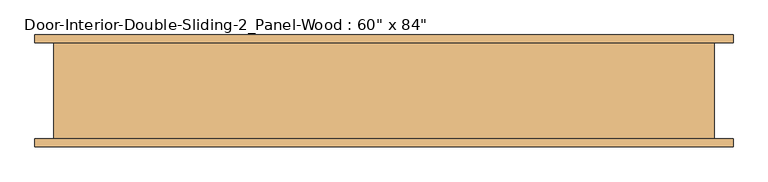
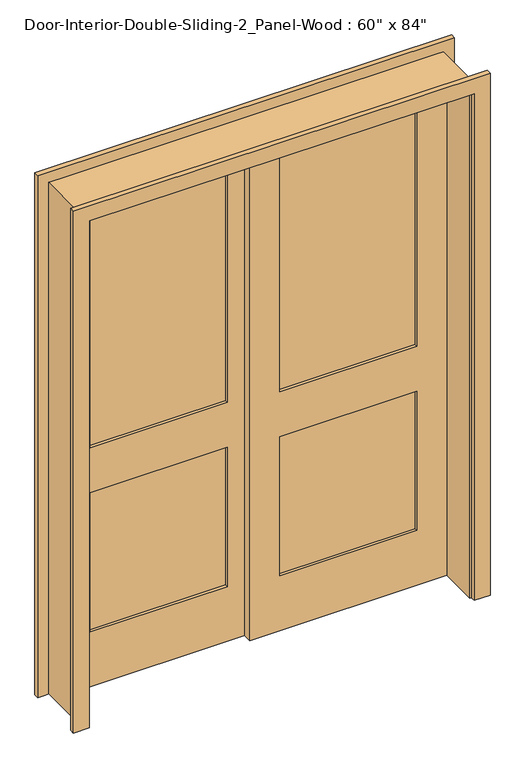
"""IFC4 building model written with IfcOpenShell, lengths in millimetres: door geometry."""

from ifc_helpers import new_model, si_unit, frame, origin, place, context, project, spatial, polyline, outline, extrude, source, transform, mapped, element, save


def door_2b3f2951(model_context):
    return source(origin(), model_context, "Body", "SweptSolid", [
        extrude(outline(polyline([(0.0, 762.0), (0.0, 787.4), (2159.0, 787.4), (2159.0, -787.4), (0.0, -787.4), (0.0, -762.0), (2133.6, -762.0), (2133.6, 762.0), (0.0, 762.0)])), frame((0.0, -117.475, 0.0), z_axis=(0.0, 1.0, 0.0), x_axis=(0.0, 0.0, 1.0)), (0.0, 0.0, 1.0), 228.6),
        extrude(outline(polyline([(2133.6, -762.0), (0.0, -762.0), (0.0, 25.4), (2133.6, 25.4), (2133.6, -762.0)]), holes=[polyline([(2014.5375, -641.35), (2014.5375, -95.25), (1009.65, -95.25), (1009.65, -641.35), (2014.5375, -641.35)]), polyline([(819.15, -641.35), (819.15, -95.25), (231.775, -95.25), (231.775, -641.35), (819.15, -641.35)])]), frame((0.0, 76.2, 0.0), z_axis=(0.0, 1.0, 0.0), x_axis=(0.0, 0.0, 1.0)), (0.0, 0.0, 1.0), 34.925),
        extrude(outline(polyline([(-95.25, 87.8416667), (-641.35, 87.8416667), (-641.35, 99.4833333), (-95.25, 99.4833333), (-95.25, 87.8416667)])), frame((0.0, 0.0, 1009.65), z_axis=(0.0, 0.0, 1.0), x_axis=(1.0, 0.0, 0.0)), (0.0, 0.0, 1.0), 1004.8875),
        extrude(outline(polyline([(-95.25, 87.8416667), (-641.35, 87.8416667), (-641.35, 99.4833333), (-95.25, 99.4833333), (-95.25, 87.8416667)])), frame((0.0, 0.0, 231.775), z_axis=(0.0, 0.0, 1.0), x_axis=(1.0, 0.0, 0.0)), (0.0, 0.0, 1.0), 587.375),
        extrude(outline(polyline([(2133.6, -25.4), (0.0, -25.4), (0.0, 762.0), (2133.6, 762.0), (2133.6, -25.4)]), holes=[polyline([(2014.5375, 95.25), (2014.5375, 641.35), (1009.65, 641.35), (1009.65, 95.25), (2014.5375, 95.25)]), polyline([(819.15, 95.25), (819.15, 641.35), (231.775, 641.35), (231.775, 95.25), (819.15, 95.25)])]), frame((0.0, 41.275, 0.0), z_axis=(0.0, 1.0, 0.0), x_axis=(0.0, 0.0, 1.0)), (0.0, 0.0, 1.0), 34.925),
        extrude(outline(polyline([(641.35, 52.9166667), (95.25, 52.9166667), (95.25, 64.5583333), (641.35, 64.5583333), (641.35, 52.9166667)])), frame((0.0, 0.0, 1009.65), z_axis=(0.0, 0.0, 1.0), x_axis=(1.0, 0.0, 0.0)), (0.0, 0.0, 1.0), 1004.8875),
        extrude(outline(polyline([(641.35, 52.9166667), (95.25, 52.9166667), (95.25, 64.5583333), (641.35, 64.5583333), (641.35, 52.9166667)])), frame((0.0, 0.0, 231.775), z_axis=(0.0, 0.0, 1.0), x_axis=(1.0, 0.0, 0.0)), (0.0, 0.0, 1.0), 587.375),
        extrude(outline(polyline([(0.0, 768.35), (0.0, 831.85), (2203.45, 831.85), (2203.45, -831.85), (0.0, -831.85), (0.0, -768.35), (2139.95, -768.35), (2139.95, 768.35), (0.0, 768.35)])), frame((0.0, 111.125, 0.0), z_axis=(0.0, 1.0, 0.0), x_axis=(0.0, 0.0, 1.0)), (0.0, 0.0, 1.0), 19.05),
        extrude(outline(polyline([(0.0, 768.35), (0.0, 831.85), (2203.45, 831.85), (2203.45, -831.85), (0.0, -831.85), (0.0, -768.35), (2139.95, -768.35), (2139.95, 768.35), (0.0, 768.35)])), frame((0.0, -136.525, 0.0), z_axis=(0.0, 1.0, 0.0), x_axis=(0.0, 0.0, 1.0)), (0.0, 0.0, 1.0), 19.05),
    ])


if __name__ == "__main__":
    model = new_model("IFC4")
    model_context = context("Model", 3, world=origin())
    ifc_project = project(units=[si_unit("LENGTHUNIT", "METRE", prefix="MILLI")], contexts=[model_context])
    site = spatial("IfcSite", under=ifc_project)
    building = spatial("IfcBuilding", under=site)
    placement = place(None, origin())
    door_shape = door_2b3f2951(model_context)
    element("IfcDoor", 1, ObjectType="Door-Interior-Double-Sliding-2_Panel-Wood : 60\" x 84\"", at=placement, inside=building, context=model_context, shape_type="MappedRepresentation", body=[
        mapped(door_shape, transform((0.0, 0.0, 0.0), x_axis=(1.0, 0.0, 0.0), y_axis=(0.0, 1.0, 0.0), z_axis=(0.0, 0.0, 1.0))),
    ])
    save(model, "model.ifc")

# Revit data of these elements
# Type "Door-Interior-Double-Sliding-2_Panel-Wood : 60\" x 84\""
#   Type Mark = "10"
#   Assembly Code = "C1020300"
#   Analytic Construction = "Wooden"
#   Top Rail = 0' - 4 11/16"
#   Thickness = 0' - 1 3/8"
#   Thermal Resistance (R) = 2.5876 (h·ft²·°F)/BTU
#   Stiles = 0' - 4 3/4"
#   Rough Width = 5' - 2"
#   Rough Height = 7' - 1"
#   Lock Rail = 0' - 7 1/2"
#   Height = 7' - 0"
#   Width = 5' - 0"
#   Heat Transfer Coefficient (U) = 0.3865 BTU/(h·ft²·°F)
#   Bottom Rail = 0' - 9 1/8"
#   Trim Material = Cherry
#   Panel Material = Cherry
#   Frame Material = Cherry
#   Visual Light Transmittance = 0
#   Solar Heat Gain Coefficient = 0
#   Wall Closure = (empty or 0)
#   Function = (empty or 0)
# Element 1 (IfcDoor, "Door-Interior-Double-Sliding-2_Panel-Wood : 60\" x 84\"")
#   Materials on its faces: "Cherry"
# Materials
#   "Cherry": class "Wood", colour RGB 226 177 128, transparency 0, Description = "Prunus Serotina", Cost = 0
